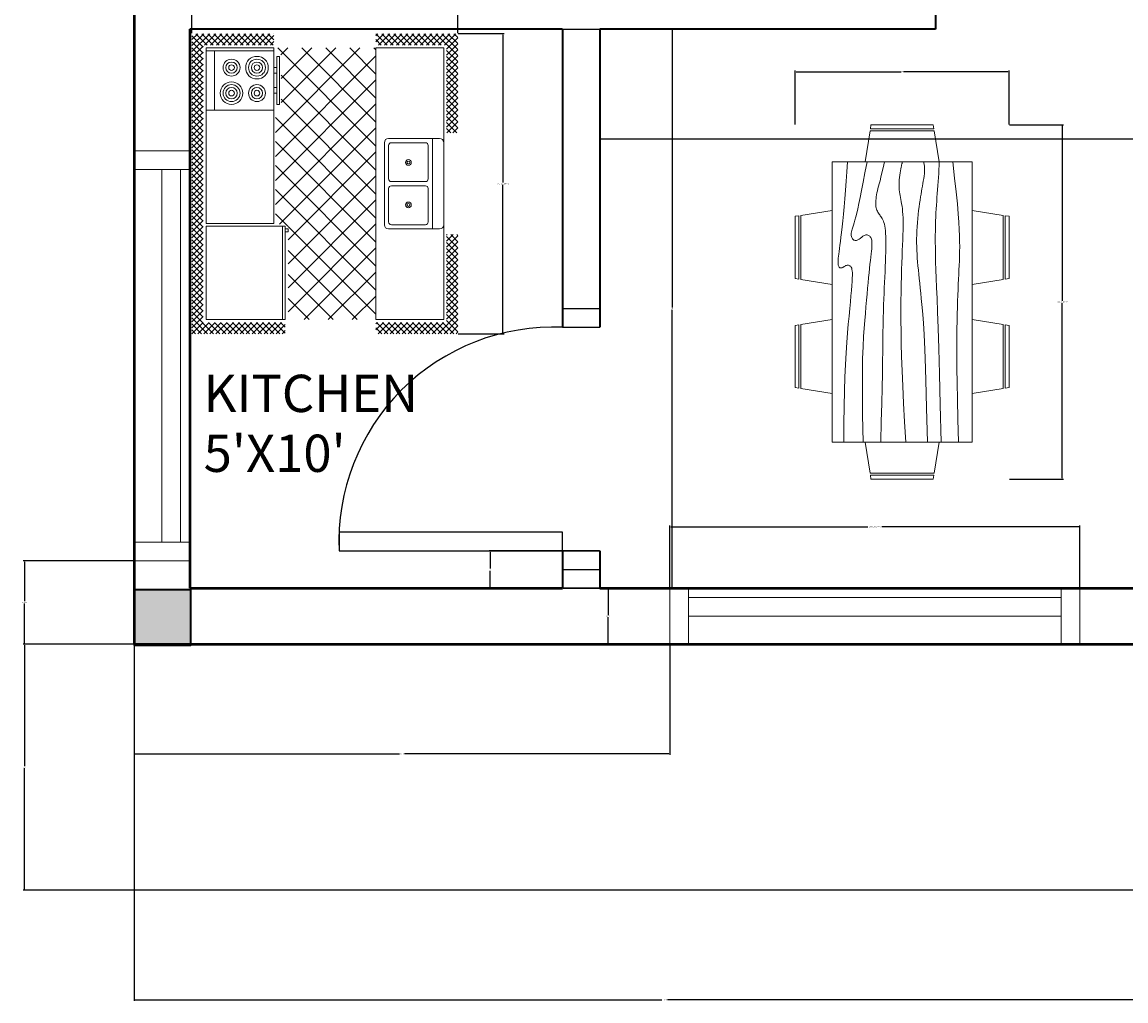
# Model space of a CAD drawing. Units: inches. Extents: x 2421 to 2780, y 382 to 769.
# Tile 1 of 4: x 2421 to 2599, y 382 to 539. Entities that reach past the tile are written whole.
import ezdxf

# ---------------------------------------------------------------- set-up
doc = ezdxf.new("R2010")
doc.units = ezdxf.units.IN
for name, color, linetype, lineweight in [('A-ANNO-DIMS', 2, 'Continuous', 18), ('A-AREA-IDEN', 7, 'Continuous', 25), ('A-COLS', 1, 'Continuous', 35), ('A-FLOR-FIXT', 3, 'Continuous', 18), ('DOOR', 1, 'Continuous', 25), ('FURNITURE', 3, 'Continuous', 18), ('INNER WALL', 2, 'Continuous', 35), ('OUTER WALL', 4, 'Continuous', 50), ('WINDOW', 5, 'Continuous', 18)]:
    doc.layers.add(name, color=color, linetype=linetype, lineweight=lineweight)
doc.styles.get("Standard").update_dxf_attribs({"font": 'arial.ttf'})
doc.dimstyles.get("Standard").update_dxf_attribs({"dimtxt": 0.18, "dimasz": 0.18, "dimexe": 0.18, "dimexo": 0.0625, "dimgap": 0.09, "dimtad": 0, "dimtih": 1, "dimtoh": 1, "dimdec": 4, "dimzin": 0, "dimdsep": 46, "dimtxsty": 'Standard', "dimcen": 0.09, "dimadec": 0, "dimazin": 0, "dimtfac": 1, "dimtdec": 4, "dimtofl": 0, "dimtmove": 0, "dimatfit": 3, "dimfxl": 1, "dimtolj": 1, "dimtzin": 0, "dimarcsym": 0})

# ---------------------------------------------------------------- blocks, each defined once
blk = doc.blocks.new('Dining Set - 36 x 72 in.')
for p, q in [((-22.2343, 26.00059), (-23.4847, 17.99762)), ((-22.2304, 26), (-5.7608, 26)), ((-22, 27.5), (-22.1562, 26.50042)), ((-5.8416, 26.5), (-22.1534, 26.5)), ((-22, 27.5), (-6, 27.5)), ((-5.8437, 26.49966), (-6, 27.5)), ((-4.5152, 17.99762), (-5.7655, 25.99926)), ((5.7657, 26.00059), (4.5153, 17.99762)), ((5.7696, 26), (22.2392, 26)), ((6, 27.5), (5.8438, 26.50042)), ((22.1584, 26.5), (5.8466, 26.5)), ((6, 27.5), (22, 27.5)), ((22.1563, 26.49966), (22, 27.5)), ((23.4848, 17.99762), (22.2345, 25.99926)), ((36, 18), (-36, 18)), ((-36, 18), (-36, -18)), ((36, -18), (36, 18)), ((-44.0006, 8.23428), (-35.9976, 9.48474)), ((44.0006, 8.23428), (35.9976, 9.48474)), ((-45.5, 8), (-44.5004, 8.15617)), ((-45.5, 8), (-45.5, -8)), ((-44.5, -8.15843), (-44.5, 8.15338)), ((-44, 8.23041), (-44, -8.23915)), ((44, 8.23041), (44, -8.23915)), ((44.5, -8.15843), (44.5, 8.15338)), ((45.5, 8), (44.5005, 8.15617)), ((45.5, 8), (45.5, -8)), ((-44.4997, -8.15631), (-45.5, -8)), ((-35.9976, -9.48476), (-43.9993, -8.2345)), ((35.9976, -9.48476), (43.9993, -8.2345)), ((44.4997, -8.15631), (45.5, -8)), ((-36, -18), (36, -18)), ((-22.2343, -26.0006), (-23.4847, -17.99762)), ((-4.5152, -17.99762), (-5.7655, -25.99928)), ((5.7657, -26.0006), (4.5153, -17.99762)), ((23.4848, -17.99762), (22.2345, -25.99928)), ((-22.2304, -26), (-5.7608, -26)), ((-22, -27.5), (-22.1562, -26.50044)), ((-5.8416, -26.5), (-22.1534, -26.5)), ((-22, -27.5), (-6, -27.5)), ((-5.8437, -26.49967), (-6, -27.5)), ((5.7696, -26), (22.2392, -26)), ((6, -27.5), (5.8438, -26.50044)), ((22.1584, -26.5), (5.8466, -26.5)), ((6, -27.5), (22, -27.5)), ((22.1563, -26.49967), (22, -27.5))]:
    blk.add_line(p, q)
for points in [[(-36, 15), (-31.1772, 14.97754), (-26.8079, 14.91406), (-22.8538, 14.81543), (-19.276, 14.6875), (-16.0362, 14.53613), (-13.0957, 14.36718), (-10.4159, 14.18652), (-7.9583, 14), (-5.6904, 13.81315), (-3.6035, 13.63021), (-1.6954, 13.45508), (0.0365, 13.29166), (1.5945, 13.14388), (2.9811, 13.01562), (4.1988, 12.9108), (5.25, 12.83333), (6.1393, 12.78613), (6.8802, 12.76823), (7.4883, 12.77767), (7.9792, 12.8125), (8.3685, 12.87077), (8.6719, 12.95052), (8.9049, 13.0498), (9.0833, 13.16666), (9.2205, 13.29899), (9.3216, 13.44401), (9.3895, 13.59879), (9.4271, 13.76041), (9.4373, 13.92594), (9.4232, 14.09245), (9.3875, 14.257), (9.3333, 14.41666), (9.2638, 14.56917), (9.1836, 14.71484), (9.0975, 14.85465), (9.0104, 14.98958), (8.9272, 15.1206), (8.8529, 15.2487), (8.7922, 15.37483), (8.75, 15.5), (8.7305, 15.62467), (8.7344, 15.74739), (8.7617, 15.86621), (8.8125, 15.97916), (8.8867, 16.08431), (8.9844, 16.17968), (9.1055, 16.26334), (9.25, 16.33333), (9.4189, 16.38802), (9.6172, 16.42708), (9.8506, 16.45052), (10.125, 16.45833), (10.4463, 16.45052), (10.8203, 16.42708), (11.2529, 16.38802), (11.75, 16.33333), (12.3184, 16.26318), (12.9694, 16.17838), (13.7151, 16.07991), (14.5677, 15.96875), (15.5395, 15.84586), (16.6426, 15.71224), (17.8893, 15.56884), (19.2917, 15.41666), (20.859, 15.25667), (22.5879, 15.08984), (24.4721, 14.91715), (26.5052, 14.73958), (28.6809, 14.5581), (30.9929, 14.3737), (33.4347, 14.18733), (36, 14)], [(-36, 10), (-28.9766, 10.14274), (-23.1725, 10.20442), (-18.4241, 10.19775), (-14.5677, 10.13541), (-11.4399, 10.03011), (-8.877, 9.89453), (-6.7154, 9.74137), (-4.7917, 9.58333), (-2.9698, 9.43082), (-1.2246, 9.28515), (0.4415, 9.14534), (2.026, 9.01041), (3.5266, 8.87939), (4.9408, 8.7513), (6.266, 8.62516), (7.5, 8.5), (8.6411, 8.37549), (9.6914, 8.2539), (10.6538, 8.13818), (11.5312, 8.03125), (12.3267, 7.93603), (13.043, 7.85547), (13.6831, 7.79248), (14.25, 7.75), (14.7471, 7.7303), (15.1797, 7.73307), (15.5537, 7.75732), (15.875, 7.80208), (16.1494, 7.86637), (16.3828, 7.94922), (16.5811, 8.04964), (16.75, 8.16666), (16.8944, 8.29915), (17.0143, 8.44531), (17.1089, 8.60319), (17.1771, 8.77083), (17.218, 8.94629), (17.2305, 9.1276), (17.2137, 9.31282), (17.1667, 9.5), (17.0895, 9.6875), (16.987, 9.875), (16.8649, 10.0625), (16.7292, 10.25), (16.5856, 10.4375), (16.4401, 10.625), (16.2985, 10.8125), (16.1667, 11), (16.05, 11.18733), (15.9518, 11.3737), (15.8752, 11.5581), (15.8229, 11.73958), (15.798, 11.91715), (15.8034, 12.08984), (15.842, 12.25667), (15.9167, 12.41666), (16.0295, 12.56836), (16.1784, 12.70833), (16.3605, 12.83268), (16.5729, 12.9375), (16.8127, 13.01888), (17.0768, 13.07291), (17.3625, 13.0957), (17.6667, 13.08333), (17.9894, 13.03312), (18.3418, 12.94726), (18.7382, 12.82918), (19.1927, 12.68229), (19.7195, 12.51001), (20.3327, 12.31575), (21.0465, 12.10294), (21.875, 11.875), (22.8357, 11.63354), (23.959, 11.37304), (25.2786, 11.08618), (26.8282, 10.76562), (28.6414, 10.40405), (30.752, 9.99414), (33.1936, 9.52856), (36, 9)], [(-36, 5.5), (-30.7157, 5.3348), (-26.069, 5.20963), (-21.9946, 5.11767), (-18.4271, 5.05208), (-15.3009, 5.00602), (-12.5508, 4.97265), (-10.1112, 4.94515), (-7.9167, 4.91666), (-5.909, 4.88167), (-4.0586, 4.83984), (-2.3429, 4.79215), (-0.7396, 4.73958), (0.7739, 4.6831), (2.22, 4.6237), (3.6213, 4.56233), (5, 4.5), (6.373, 4.43782), (7.7344, 4.3776), (9.0723, 4.32129), (10.375, 4.27083), (11.6309, 4.22819), (12.8281, 4.19531), (13.9551, 4.17415), (15, 4.16666), (15.954, 4.17448), (16.819, 4.19791), (17.6001, 4.23698), (18.3021, 4.29166), (18.9299, 4.36198), (19.4883, 4.44791), (19.9823, 4.54948), (20.4167, 4.66666), (20.7969, 4.79899), (21.1302, 4.94401), (21.4245, 5.09879), (21.6875, 5.26041), (21.9271, 5.42594), (22.1511, 5.59245), (22.3672, 5.757), (22.5834, 5.91666), (22.8065, 6.06868), (23.0404, 6.21093), (23.2879, 6.34147), (23.5521, 6.45833), (23.8358, 6.55957), (24.142, 6.64323), (24.4735, 6.70735), (24.8334, 6.75), (25.2235, 6.76969), (25.642, 6.76692), (26.0858, 6.74267), (26.5521, 6.69791), (27.0379, 6.63362), (27.5404, 6.55078), (28.0565, 6.45036), (28.5834, 6.33333), (29.1242, 6.19987), (29.7071, 6.04687), (30.3661, 5.87044), (31.1354, 5.66666), (32.0493, 5.43164), (33.142, 5.16146), (34.4475, 4.85221), (36, 4.5)], [(-36, -1), (-30.7915, -0.6591), (-26.0195, -0.38216), (-21.6519, -0.16284), (-17.6563, 0.00521), (-14.0005, 0.12833), (-10.6523, 0.21289), (-7.5796, 0.26522), (-4.75, 0.29166), (-2.134, 0.29793), (0.2878, 0.28711), (2.5317, 0.26163), (4.6146, 0.22396), (6.5529, 0.17651), (8.3633, 0.12174), (10.0623, 0.06209), (11.6667, 0), (13.1899, -0.06201), (14.6341, -0.1211), (15.9982, -0.17432), (17.2813, -0.21875), (18.4823, -0.25147), (19.6003, -0.26953), (20.6343, -0.27002), (21.5834, -0.25), (22.4481, -0.20768), (23.2357, -0.14584), (23.9549, -0.06836), (24.6146, 0.02083), (25.2235, 0.11784), (25.7904, 0.21875), (26.3241, 0.31966), (26.8334, 0.41666), (27.3265, 0.50618), (27.8099, 0.58593), (28.2894, 0.65397), (28.7709, 0.70833), (29.2601, 0.74707), (29.763, 0.76823), (30.2855, 0.76985), (30.8334, 0.75), (31.4088, 0.70784), (31.9994, 0.64713), (32.589, 0.57275), (33.1615, 0.48958), (33.7008, 0.4025), (34.1908, 0.3164), (34.6153, 0.23616), (34.9584, 0.16666), (35.2099, 0.11165), (35.3848, 0.07031), (35.504, 0.04069), (35.5886, 0.02083), (35.6594, 0.00879), (35.7377, 0.0026), (35.8442, 0.00032), (36, 0)], [(-36, -6.5), (-27.1843, -6.31267), (-20.084, -6.1263), (-14.469, -5.9419), (-10.1094, -5.76042), (-6.7752, -5.58285), (-4.2363, -5.41016), (-2.2629, -5.24333), (-0.625, -5.08334), (0.8708, -4.93099), (2.2715, -4.78646), (3.5872, -4.64974), (4.8281, -4.52084), (6.0046, -4.39974), (7.127, -4.28646), (8.2053, -4.18099), (9.25, -4.08334), (10.2705, -3.99382), (11.2734, -3.91407), (12.2647, -3.84603), (13.25, -3.79167), (14.2354, -3.75293), (15.2266, -3.73177), (16.2295, -3.73015), (17.25, -3.75), (18.2912, -3.79248), (19.3451, -3.85547), (20.4009, -3.93604), (21.4479, -4.03125), (22.4754, -4.13819), (23.4727, -4.25391), (24.4289, -4.37549), (25.3334, -4.5), (26.1785, -4.62492), (26.9694, -4.74935), (27.7145, -4.87281), (28.4219, -4.99479), (29.1, -5.11483), (29.7572, -5.23242), (30.4016, -5.34709), (31.0417, -5.45834), (31.6837, -5.56437), (32.3262, -5.65821), (32.9658, -5.73153), (33.599, -5.77604), (34.2224, -5.78345), (34.8327, -5.74545), (35.4264, -5.65373), (36, -5.5)], [(-36, -10), (-26.4022, -9.81299), (-18.4675, -9.62891), (-11.9839, -9.45069), (-6.7396, -9.28125), (-2.5226, -9.12354), (0.8789, -8.98047), (3.6769, -8.85498), (6.0833, -8.75), (8.2767, -8.66765), (10.3021, -8.60677), (12.1712, -8.56543), (13.8958, -8.54167), (15.4876, -8.53353), (16.9583, -8.53907), (18.3197, -8.55632), (19.5834, -8.58334), (20.7616, -8.61841), (21.8685, -8.66081), (22.9188, -8.71004), (23.9271, -8.76563), (24.9081, -8.82707), (25.8763, -8.89388), (26.8465, -8.96558), (27.8334, -9.04167), (28.8474, -9.12118), (29.8828, -9.20117), (30.93, -9.27824), (31.9792, -9.34896), (33.0205, -9.40991), (34.0443, -9.45768), (35.0407, -9.48885), (36, -9.5)], [(-36, -14.5), (-30.0881, -14.33513), (-25.0332, -14.21224), (-20.7312, -14.12647), (-17.0781, -14.07292), (-13.97, -14.04671), (-11.3027, -14.04297), (-8.9724, -14.05681), (-6.875, -14.08334), (-4.9224, -14.11833), (-3.0905, -14.16016), (-1.3709, -14.20785), (0.2448, -14.26042), (1.7647, -14.3169), (3.1973, -14.3763), (4.5507, -14.43767), (5.8333, -14.5), (7.0554, -14.5621), (8.235, -14.62175), (9.3922, -14.67652), (10.5469, -14.72396), (11.7192, -14.76164), (12.929, -14.78711), (14.1965, -14.79794), (15.5417, -14.79167), (16.9933, -14.76424), (18.6152, -14.70508), (20.4804, -14.60197), (22.6615, -14.44271), (25.2312, -14.21509), (28.2624, -13.9069), (31.8277, -13.50594), (36, -13)]]:
    blk.add_lwpolyline(points)
blk = doc.blocks.new('Kitchen Layout - 7 x 8 ft')
for p, q in [((-5, 81.32), (2.68, 89)), ((-5, 83.44), (0.56, 89)), ((-5, 85.56), (-1.56, 89)), ((-5, 87.68), (-3.68, 89)), ((-1, 84.97), (-5, 88.97)), ((-1, 82.85), (-5, 86.85)), ((1.09, 85), (-2.91, 89)), ((3.21, 85), (-0.79, 89)), ((0.81, 85), (4.81, 89)), ((5.34, 85), (1.34, 89)), ((2.93, 85), (6.93, 89)), ((7.46, 85), (3.46, 89)), ((5.05, 85), (9.05, 89)), ((9.58, 85), (5.58, 89)), ((7.17, 85), (11.17, 89)), ((11.7, 85), (7.7, 89)), ((9.29, 85), (13.29, 89)), ((13.82, 85), (9.82, 89)), ((11.41, 85), (15.41, 89)), ((15.94, 85), (11.94, 89)), ((13.53, 85), (17.53, 89)), ((18.06, 85), (14.06, 89)), ((15.65, 85), (19.65, 89)), ((20.18, 85), (16.18, 89)), ((17.78, 85), (21.78, 89)), ((22.31, 85), (18.31, 89)), ((19.9, 85), (23.9, 89)), ((24.43, 85), (20.43, 89)), ((22.02, 85), (26.02, 89)), ((26.55, 85), (22.55, 89)), ((24.14, 85), (28.14, 89)), ((28.67, 85), (24.67, 89)), ((26.26, 85), (30.26, 89)), ((30.79, 85), (26.79, 89)), ((28.38, 85), (32.38, 89)), ((32.91, 85), (28.91, 89)), ((30.5, 85), (34.5, 89)), ((35.03, 85), (31.03, 89)), ((32.63, 85), (36.63, 89)), ((37.16, 85), (33.16, 89)), ((34.75, 85), (38.75, 89)), ((39.28, 85), (35.28, 89)), ((36.87, 85), (40.87, 89)), ((41.4, 85), (37.4, 89)), ((38.99, 85), (42.99, 89)), ((43.52, 85), (39.52, 89)), ((41.11, 85), (45.11, 89)), ((45.64, 85), (41.64, 89)), ((43.23, 85), (47.23, 89)), ((47.76, 85), (43.76, 89)), ((45.35, 85), (49.35, 89)), ((49.88, 85), (45.88, 89)), ((47.47, 85), (51.47, 89)), ((52, 85), (48, 89)), ((49.6, 85), (53.6, 89)), ((54.13, 85), (50.13, 89)), ((51.72, 85), (55.72, 89)), ((56.25, 85), (52.25, 89)), ((53.84, 85), (57.84, 89)), ((58.37, 85), (54.37, 89)), ((55.96, 85), (59.96, 89)), ((60.49, 85), (56.49, 89)), ((58.08, 85), (62.08, 89)), ((62.61, 85), (58.61, 89)), ((60.2, 85), (64.2, 89)), ((64.73, 85), (60.73, 89)), ((62.32, 85), (66.32, 89)), ((66.85, 85), (62.85, 89)), ((64.45, 85), (68.45, 89)), ((68.97, 85), (64.97, 89)), ((66.57, 85), (70.57, 89)), ((71.1, 85), (67.1, 89)), ((68.69, 85), (72.69, 89)), ((73.22, 85), (69.22, 89)), ((70.81, 85), (74.81, 89)), ((75.34, 85), (71.34, 89)), ((72.93, 85), (76.93, 89)), ((77.46, 85), (73.46, 89)), ((75.05, 85), (79.05, 89)), ((79.58, 85), (75.58, 89)), ((77.17, 85), (81.17, 89)), ((81.7, 85), (77.7, 89)), ((79.29, 85), (83.29, 89)), ((83.82, 85), (79.82, 89)), ((81.42, 85), (85.42, 89)), ((85.95, 85), (81.95, 89)), ((83.54, 85), (87.54, 89)), ((88.07, 85), (84.07, 89)), ((85.66, 85), (89.66, 89)), ((90.19, 85), (86.19, 89)), ((87.78, 85), (91.78, 89)), ((92.31, 85), (88.31, 89)), ((89.9, 85), (93.9, 89)), ((94.43, 85), (90.43, 89)), ((92.02, 85), (96.02, 89)), ((96.55, 85), (92.55, 89)), ((94.14, 85), (98.14, 89)), ((101, 82.67), (94.67, 89)), ((96.27, 85), (100.27, 89)), ((101, 84.79), (96.79, 89)), ((97, 83.61), (101, 87.61)), ((101, 86.92), (98.92, 89)), ((-1, 80.73), (-5, 84.73)), ((-5, 79.19), (-1, 83.19)), ((-1, 78.61), (-5, 82.61)), ((34, 84), (96, 84)), ((34, 60), (34, 84)), ((96, 84), (96, 60)), ((97, 81.49), (101, 85.49)), ((101, 80.55), (97, 84.55)), ((97, 79.37), (101, 83.37)), ((101, 78.43), (97, 82.43)), ((-5, 77.07), (-1, 81.07)), ((-1, 76.49), (-5, 80.49)), ((-5, 74.95), (-1, 78.95)), ((-1, 74.36), (-5, 78.36)), ((74, 81), (95, 81)), ((97, 77.25), (101, 81.25)), ((101, 76.31), (97, 80.31)), ((97, 75.13), (101, 79.13)), ((101, 74.19), (97, 78.19)), ((-5, 72.83), (-1, 76.83)), ((-1, 72.24), (-5, 76.24)), ((-5, 70.71), (-1, 74.71)), ((-1, 70.12), (-5, 74.12)), ((97, 73.01), (101, 77.01)), ((101, 72.07), (97, 76.07)), ((97, 70.89), (101, 74.89)), ((-5, 68.59), (-1, 72.59)), ((-1, 68), (-5, 72)), ((-5, 66.47), (-1, 70.47)), ((101, 69.95), (97, 73.95)), ((97, 68.76), (101, 72.76)), ((101, 67.82), (97, 71.82)), ((97, 66.64), (101, 70.64)), ((-1, 65.88), (-5, 69.88)), ((-5, 64.35), (-1, 68.35)), ((-1, 63.76), (-5, 67.76)), ((101, 65.7), (97, 69.7)), ((97, 64.52), (101, 68.52)), ((101, 63.58), (97, 67.58)), ((97, 62.4), (101, 66.4)), ((-5, 62.22), (-1, 66.22)), ((-1, 61.64), (-5, 65.64)), ((-5, 60.1), (-1, 64.1)), ((-1, 59.52), (-5, 63.52)), ((101, 61.46), (97, 65.46)), ((97, 60.28), (101, 64.28)), ((100.34, 60), (97, 63.34)), ((-5, 57.98), (-1, 61.98)), ((-1, 57.39), (-5, 61.39)), ((-1.73, 56), (-5, 59.27)), ((-4.86, 56), (-1, 59.86)), ((10.4, 24), (45.9, 59.5)), ((18.88, 24), (54.38, 59.5)), ((27.37, 24), (62.87, 59.5)), ((33.03, 55.11), (37.41, 59.5)), ((96, 60), (34, 60)), ((35.85, 24), (71.35, 59.5)), ((76.2, 24), (40.7, 59.5)), ((84.68, 24), (49.18, 59.5)), ((93.17, 24), (57.67, 59.5)), ((61.31, 24), (96, 58.69)), ((96, 29.65), (66.15, 59.5)), ((80, 60), (80, 59)), ((82, 59), (82, 60)), ((87, 59), (87, 60)), ((89, 60), (89, 59)), ((98.22, 60), (97, 61.22)), ((98.84, 60), (101, 62.16)), ((100.96, 60), (101, 60.04)), ((-3.85, 56), (-5, 57.15)), ((-2.74, 56), (-1, 57.74)), ((0, 57), (33, 57)), ((0, 30.57), (24.43, 55)), ((0, 39.06), (15.94, 55)), ((0, 47.54), (7.46, 55)), ((1.91, 24), (32.91, 55)), ((33.77, 24), (2.77, 55)), ((42.26, 24), (11.26, 55)), ((50.74, 24), (19.74, 55)), ((59.23, 24), (28.23, 55)), ((31, 55), (31, 56)), ((32, 55), (31, 55)), ((32, 56), (32, 55)), ((67.71, 24), (33.68, 58.04)), ((44.34, 24), (77.84, 57.5)), ((52.82, 24), (86.32, 57.5)), ((96, 38.14), (76.64, 57.5)), ((96, 46.63), (85.13, 57.5)), ((96, 55.11), (93.57, 57.54)), ((25.29, 24), (0, 49.29)), ((69.79, 24), (96, 50.21)), ((16.8, 24), (0, 40.8)), ((78.28, 24), (96, 41.72)), ((8.32, 24), (0, 32.32)), ((86.76, 24), (96, 33.24)), ((-5, 21.92), (-2.92, 24)), ((-5, 19.8), (-1, 23.8)), ((-1, 21.33), (-3.67, 24)), ((-1, 23.45), (-1.55, 24)), ((0, 24), (96, 24)), ((0, 0), (0, 24)), ((95.25, 24), (96, 24.75)), ((96, 24), (96, 0)), ((97, 22.1), (98.9, 24)), ((97, 19.97), (101, 23.97)), ((101, 21.16), (98.16, 24)), ((101, 23.28), (100.28, 24)), ((-1, 19.21), (-5, 23.21)), ((-5, 17.68), (-1, 21.68)), ((-1, 17.09), (-5, 21.09)), ((-5, 15.55), (-1, 19.55)), ((101, 19.03), (97, 23.03)), ((97, 17.85), (101, 21.85)), ((101, 16.91), (97, 20.91)), ((97, 15.73), (101, 19.73)), ((-1, 14.97), (-5, 18.97)), ((-5, 13.43), (-1, 17.43)), ((-1, 12.85), (-5, 16.85)), ((47.25, 6.5), (47.25, 18.5)), ((48.75, 18.5), (48.75, 6.5)), ((101, 14.79), (97, 18.79)), ((97, 13.61), (101, 17.61)), ((101, 12.67), (97, 16.67)), ((-5, 11.31), (-1, 15.31)), ((-1, 10.73), (-5, 14.73)), ((-5, 9.19), (-1, 13.19)), ((-1, 8.6), (-5, 12.6)), ((97, 11.49), (101, 15.49)), ((101, 10.55), (97, 14.55)), ((97, 9.37), (101, 13.37)), ((101, 8.43), (97, 12.43)), ((-5, 7.07), (-1, 11.07)), ((-1, 6.48), (-5, 10.48)), ((-5, 4.95), (-1, 8.95)), ((-1, 4.36), (-5, 8.36)), ((97, 7.25), (101, 11.25)), ((101, 6.31), (97, 10.31)), ((97, 5.12), (101, 9.12)), ((101, 4.18), (97, 8.18)), ((-5, 2.83), (-1, 6.83)), ((-1, 2.24), (-5, 6.24)), ((-5, 0.71), (-1, 4.71)), ((-1, 0.12), (-5, 4.12)), ((64, 4), (32, 4)), ((97, 3), (101, 7)), ((101, 2.06), (97, 6.06)), ((97, 0.88), (101, 4.88)), ((101, -0.06), (97, 3.94)), ((-5, -1.42), (-1, 2.58)), ((2, -5), (-5, 2)), ((-5, -3.54), (-1, 0.46)), ((96, 0), (0, 0)), ((93.24, -5), (101, 2.76)), ((95.36, -5), (101, 0.64)), ((101, -2.18), (97, 1.82)), ((-0.12, -5), (-5, -0.12)), ((-2.25, -5), (-5, -2.25)), ((-4.34, -5), (-0.34, -1)), ((-2.22, -5), (1.78, -1)), ((-0.1, -5), (3.9, -1)), ((4.12, -5), (0.12, -1)), ((2.02, -5), (6.02, -1)), ((6.24, -5), (2.24, -1)), ((4.14, -5), (8.14, -1)), ((8.36, -5), (4.36, -1)), ((6.27, -5), (10.27, -1)), ((10.48, -5), (6.48, -1)), ((8.39, -5), (12.39, -1)), ((12.6, -5), (8.6, -1)), ((10.51, -5), (14.51, -1)), ((14.73, -5), (10.73, -1)), ((12.63, -5), (16.63, -1)), ((16.85, -5), (12.85, -1)), ((14.75, -5), (18.75, -1)), ((18.97, -5), (14.97, -1)), ((16.87, -5), (20.87, -1)), ((21.09, -5), (17.09, -1)), ((18.99, -5), (22.99, -1)), ((23.21, -5), (19.21, -1)), ((21.11, -5), (25.11, -1)), ((25.33, -5), (21.33, -1)), ((23.24, -5), (27.24, -1)), ((27.45, -5), (23.45, -1)), ((25.36, -5), (29.36, -1)), ((29.57, -5), (25.57, -1)), ((27.48, -5), (30, -2.48)), ((30, -3.3), (27.7, -1)), ((30, -1.18), (29.82, -1)), ((66, -2.54), (67.54, -1)), ((66, -4.66), (69.66, -1)), ((69.88, -5), (66, -1.12)), ((67.76, -5), (66, -3.24)), ((67.78, -5), (71.78, -1)), ((72, -5), (68, -1)), ((69.9, -5), (73.9, -1)), ((74.12, -5), (70.12, -1)), ((72.03, -5), (76.03, -1)), ((76.24, -5), (72.24, -1)), ((74.15, -5), (78.15, -1)), ((78.36, -5), (74.36, -1)), ((76.27, -5), (80.27, -1)), ((80.49, -5), (76.49, -1)), ((78.39, -5), (82.39, -1)), ((82.61, -5), (78.61, -1)), ((80.51, -5), (84.51, -1)), ((84.73, -5), (80.73, -1)), ((82.63, -5), (86.63, -1)), ((86.85, -5), (82.85, -1)), ((84.75, -5), (88.75, -1)), ((88.97, -5), (84.97, -1)), ((86.88, -5), (90.88, -1)), ((91.09, -5), (87.09, -1)), ((89, -5), (93, -1)), ((93.21, -5), (89.21, -1)), ((91.12, -5), (95.12, -1)), ((95.34, -5), (91.34, -1)), ((97.46, -5), (93.46, -1)), ((99.58, -5), (95.58, -1)), ((101, -4.3), (97, -0.3)), ((97.48, -5), (101, -1.48)), ((99.6, -5), (101, -3.6)), ((-4.37, -5), (-5, -4.37)), ((29.6, -5), (30, -4.6))]:
    blk.add_line(p, q)
for points in [[(0, 56), (0, 84), (33, 84), (33, 56)], [(74, 60), (74, 84), (95, 84), (95, 60)], [(76, 58), (76, 59), (93, 59), (93, 58)]]:
    blk.add_lwpolyline(points, close=True)
for points in [[(33.5, 21), (62.5, 21)], [(32, 1.5), (32, 19.5)], [(33.5, 6.5), (33.5, 18.5)], [(34.5, 19.5), (46.25, 19.5)], [(49.75, 19.5), (61.5, 19.5)], [(62.5, 18.5), (62.5, 6.5)], [(64, 19.5), (64, 1.5)], [(46.25, 5.5), (34.5, 5.5)], [(61.5, 5.5), (49.75, 5.5)], [(62.5, 0), (33.5, 0)]]:
    blk.add_lwpolyline(points)
for centre, radius in [((80, 75), 4), ((80, 75), 3), ((80, 75), 2), ((80, 75), 1), ((89, 75), 3), ((89, 75), 2), ((89, 75), 1), ((80, 66), 3), ((80, 66), 2), ((80, 66), 1), ((89, 66), 4), ((89, 66), 3), ((89, 66), 2), ((89, 66), 1), ((40.5, 12.5), 1), ((40.5, 12.5), 0.5), ((55.5, 12.5), 1), ((55.5, 12.5), 0.5)]:
    blk.add_circle(centre, radius)
for centre, radius, start, end in [((33.5, 19.5), 1.5, 90, 180), ((62.5, 19.5), 1.5, 0, 90), ((34.5, 18.5), 1, 90, 180), ((46.25, 18.5), 1, 0, 90), ((49.75, 18.5), 1, 90, 180), ((61.5, 18.5), 1, 0, 90), ((34.5, 6.5), 1, 180, 270), ((46.25, 6.5), 1, 270, 0), ((49.75, 6.5), 1, 180, 270), ((61.5, 6.5), 1, 270, 0), ((33.5, 1.5), 1.5, 180, 270), ((62.5, 1.5), 1.5, 270, 0)]:
    blk.add_arc(centre, radius, start, end)
blk = doc.blocks.new('DOOR-36IN-INT')
for p, q in [((0, 6), (0, 0)), ((3, 6), (3, 0)), ((39, 6), (39, 0)), ((42, 6), (42, 0))]:
    blk.add_line(p, q)
blk.add_lwpolyline([(3, 6), (6, 6), (6, 42), (3, 42)], close=True)
blk.add_arc((4.5, 7.5), 34.53, 357.5104, 92.4896)
blk = doc.blocks.new('WIN-60IN')
for p, q in [((0, 0), (0, 9)), ((3, 0), (3, 9)), ((63, 9), (63, 0)), ((66, 9), (66, 0)), ((63, 4.5), (3, 4.5)), ((63, 1.5), (3, 1.5))]:
    blk.add_line(p, q)
blk = doc.blocks.new('COL-9X9IN')
h = blk.add_hatch(color=256)
h.dxf.hatch_style = 1
h.paths.add_polyline_path([(9, 9), (0, 9), (0, 0), (9, 0)])
blk.add_lwpolyline([(0, 9), (9, 9), (9, 0), (0, 0)], close=True)
blk = doc.blocks.new('*D20')
at = {"layer": 'A-ANNO-DIMS', "color": 0, "lineweight": -2, "transparency": 16777216}
for p, q in [((2525.72, 448.24), (2525.72, 458.26)), ((2525.9, 458.08), (2557.6, 458.08)), ((2591.54, 458.08), (2559.84, 458.08)), ((2591.72, 448.24), (2591.72, 458.26))]:
    blk.add_line(p, q, dxfattribs=at)
at = {"layer": 'A-ANNO-DIMS', "color": 0, "transparency": 16777216}
for points in [[(2525.9, 458.11), (2525.9, 458.05), (2525.72, 458.08)], [(2591.54, 458.11), (2591.54, 458.05), (2591.72, 458.08)]]:
    blk.add_solid(points, dxfattribs=at)
at = {"layer": 'Defpoints', "color": 0, "transparency": 16777216}
for p in [(2525.72, 458.08), (2525.72, 448.18), (2591.72, 448.18)]:
    blk.add_point(p, dxfattribs=at)
at = {"layer": 'A-ANNO-DIMS', "color": 0, "transparency": 16777216, "insert": (2558.72, 458.08), "char_height": 0.18, "attachment_point": 5}
blk.add_mtext('\\A1;WINDOW 66 TYP.', dxfattribs=at)
blk = doc.blocks.new('*D21')
at = {"layer": 'A-ANNO-DIMS', "color": 0, "lineweight": -2, "transparency": 16777216}
for p, q in [((2525.66, 448.18), (2515.64, 448.18)), ((2515.82, 448), (2515.82, 443.86)), ((2515.82, 439.36), (2515.82, 443.5)), ((2525.66, 439.18), (2515.64, 439.18))]:
    blk.add_line(p, q, dxfattribs=at)
at = {"layer": 'A-ANNO-DIMS', "color": 0, "transparency": 16777216}
for points in [[(2515.79, 448), (2515.85, 448), (2515.82, 448.18)], [(2515.79, 439.36), (2515.85, 439.36), (2515.82, 439.18)]]:
    blk.add_solid(points, dxfattribs=at)
at = {"layer": 'Defpoints', "color": 0, "transparency": 16777216}
for p in [(2525.72, 448.18), (2515.82, 439.18), (2525.72, 439.18)]:
    blk.add_point(p, dxfattribs=at)
at = {"layer": 'A-ANNO-DIMS', "color": 0, "transparency": 16777216, "insert": (2515.82, 443.68), "char_height": 0.18, "attachment_point": 5}
blk.add_mtext('\\A1;9 TYP.', dxfattribs=at)
blk = doc.blocks.new('*D42')
at = {"layer": 'A-ANNO-DIMS', "color": 0, "lineweight": -2, "transparency": 16777216}
for p, q in [((2580.41, 522.76), (2589.08, 522.76)), ((2588.9, 522.58), (2588.9, 494.44)), ((2588.9, 465.92), (2588.9, 494.07)), ((2580.41, 465.74), (2589.08, 465.74))]:
    blk.add_line(p, q, dxfattribs=at)
at = {"layer": 'A-ANNO-DIMS', "color": 0, "transparency": 16777216}
for points in [[(2588.87, 522.58), (2588.93, 522.58), (2588.9, 522.76)], [(2588.87, 465.92), (2588.93, 465.92), (2588.9, 465.74)]]:
    blk.add_solid(points, dxfattribs=at)
at = {"layer": 'Defpoints', "color": 0, "transparency": 16777216}
for p in [(2580.34, 522.76), (2588.9, 522.76), (2580.34, 465.74)]:
    blk.add_point(p, dxfattribs=at)
at = {"layer": 'A-ANNO-DIMS', "color": 0, "transparency": 16777216, "insert": (2588.9, 494.25), "char_height": 0.18, "attachment_point": 5}
blk.add_mtext('\\A1;DINING SET 57', dxfattribs=at)
blk = doc.blocks.new('*D43')
at = {"layer": 'A-ANNO-DIMS', "color": 0, "lineweight": -2, "transparency": 16777216}
for p, q in [((2545.88, 522.83), (2545.88, 531.5)), ((2580.34, 522.83), (2580.34, 531.5)), ((2546.06, 531.32), (2562.89, 531.32)), ((2580.16, 531.32), (2563.33, 531.32))]:
    blk.add_line(p, q, dxfattribs=at)
at = {"layer": 'A-ANNO-DIMS', "color": 0, "transparency": 16777216}
for points in [[(2546.06, 531.35), (2546.06, 531.29), (2545.88, 531.32)], [(2580.16, 531.35), (2580.16, 531.29), (2580.34, 531.32)]]:
    blk.add_solid(points, dxfattribs=at)
at = {"layer": 'Defpoints', "color": 0, "transparency": 16777216}
for p in [(2545.88, 531.32), (2545.88, 522.76), (2580.34, 522.76)]:
    blk.add_point(p, dxfattribs=at)
at = {"layer": 'A-ANNO-DIMS', "color": 0, "transparency": 16777216, "insert": (2563.11, 531.32), "char_height": 0.18, "attachment_point": 5}
blk.add_mtext('\\A1;34', dxfattribs=at)
blk = doc.blocks.new('*D44')
at = {"layer": 'A-ANNO-DIMS', "color": 0, "lineweight": -2, "transparency": 16777216}
for p, q in [((2491.67, 537.44), (2499.03, 537.44)), ((2498.85, 537.26), (2498.85, 513.47)), ((2498.85, 489.32), (2498.85, 513.11)), ((2491.67, 489.14), (2499.03, 489.14))]:
    blk.add_line(p, q, dxfattribs=at)
at = {"layer": 'A-ANNO-DIMS', "color": 0, "transparency": 16777216}
for points in [[(2498.82, 537.26), (2498.88, 537.26), (2498.85, 537.44)], [(2498.82, 489.32), (2498.88, 489.32), (2498.85, 489.14)]]:
    blk.add_solid(points, dxfattribs=at)
at = {"layer": 'Defpoints', "color": 0, "transparency": 16777216}
for p in [(2491.61, 537.44), (2498.85, 537.44), (2491.61, 489.14)]:
    blk.add_point(p, dxfattribs=at)
at = {"layer": 'A-ANNO-DIMS', "color": 0, "transparency": 16777216, "insert": (2498.85, 513.29), "char_height": 0.18, "attachment_point": 5}
blk.add_mtext('\\A1;KITCHEN UNIT 48', dxfattribs=at)
blk = doc.blocks.new('*D45')
at = {"layer": 'A-ANNO-DIMS', "color": 0, "lineweight": -2, "transparency": 16777216}
for p, q in [((2448.78, 537.5), (2448.78, 544.86)), ((2448.96, 544.68), (2469.97, 544.68)), ((2491.43, 544.68), (2470.42, 544.68)), ((2491.61, 537.5), (2491.61, 544.86))]:
    blk.add_line(p, q, dxfattribs=at)
at = {"layer": 'A-ANNO-DIMS', "color": 0, "transparency": 16777216}
for points in [[(2448.96, 544.71), (2448.96, 544.65), (2448.78, 544.68)], [(2491.43, 544.71), (2491.43, 544.65), (2491.61, 544.68)]]:
    blk.add_solid(points, dxfattribs=at)
at = {"layer": 'Defpoints', "color": 0, "transparency": 16777216}
for p in [(2448.78, 544.68), (2448.78, 537.44), (2491.61, 537.44)]:
    blk.add_point(p, dxfattribs=at)
at = {"layer": 'A-ANNO-DIMS', "color": 0, "transparency": 16777216, "insert": (2470.19, 544.68), "char_height": 0.18, "attachment_point": 5}
blk.add_mtext('\\A1;43', dxfattribs=at)
blk = doc.blocks.new('*D49')
at = {"layer": 'A-ANNO-DIMS', "color": 0, "lineweight": -2, "transparency": 16777216}
for p, q in [((2439.47, 439.12), (2439.47, 381.75)), ((2610.35, 439.12), (2610.35, 381.75)), ((2439.65, 381.93), (2524.45, 381.93)), ((2610.17, 381.93), (2525.36, 381.93))]:
    blk.add_line(p, q, dxfattribs=at)
at = {"layer": 'A-ANNO-DIMS', "color": 0, "transparency": 16777216}
for points in [[(2439.65, 381.96), (2439.65, 381.9), (2439.47, 381.93)], [(2610.17, 381.96), (2610.17, 381.9), (2610.35, 381.93)]]:
    blk.add_solid(points, dxfattribs=at)
at = {"layer": 'Defpoints', "color": 0, "transparency": 16777216}
for p in [(2439.47, 439.18), (2610.35, 439.18), (2610.35, 381.93)]:
    blk.add_point(p, dxfattribs=at)
at = {"layer": 'A-ANNO-DIMS', "color": 0, "transparency": 16777216, "insert": (2524.91, 381.93), "char_height": 0.18, "attachment_point": 5}
blk.add_mtext('\\A1;170.88', dxfattribs=at)
blk = doc.blocks.new('*D50')
at = {"layer": 'A-ANNO-DIMS', "color": 0, "lineweight": -2, "transparency": 16777216}
for p, q in [((2439.4, 439.18), (2421.64, 439.18)), ((2421.82, 439), (2421.82, 419.56)), ((2421.82, 399.76), (2421.82, 419.2)), ((2610.28, 399.58), (2421.64, 399.58))]:
    blk.add_line(p, q, dxfattribs=at)
at = {"layer": 'A-ANNO-DIMS', "color": 0, "transparency": 16777216}
for points in [[(2421.79, 439), (2421.85, 439), (2421.82, 439.18)], [(2421.79, 399.76), (2421.85, 399.76), (2421.82, 399.58)]]:
    blk.add_solid(points, dxfattribs=at)
at = {"layer": 'Defpoints', "color": 0, "transparency": 16777216}
for p in [(2421.82, 439.18), (2439.47, 439.18), (2610.35, 399.58)]:
    blk.add_point(p, dxfattribs=at)
at = {"layer": 'A-ANNO-DIMS', "color": 0, "transparency": 16777216, "insert": (2421.82, 419.38), "char_height": 0.18, "attachment_point": 5}
blk.add_mtext('\\A1;39.6', dxfattribs=at)
blk = doc.blocks.new('*D51')
at = {"layer": 'A-ANNO-DIMS', "color": 0, "lineweight": -2, "transparency": 16777216}
for p, q in [((2508.53, 538.18), (2526.3, 538.18)), ((2526.12, 538), (2526.12, 493.36)), ((2526.12, 448.36), (2526.12, 493)), ((2508.53, 448.18), (2526.3, 448.18))]:
    blk.add_line(p, q, dxfattribs=at)
at = {"layer": 'A-ANNO-DIMS', "color": 0, "transparency": 16777216}
for points in [[(2526.09, 538), (2526.15, 538), (2526.12, 538.18)], [(2526.09, 448.36), (2526.15, 448.36), (2526.12, 448.18)]]:
    blk.add_solid(points, dxfattribs=at)
at = {"layer": 'Defpoints', "color": 0, "transparency": 16777216}
for p in [(2508.47, 538.18), (2508.47, 448.18), (2526.12, 448.18)]:
    blk.add_point(p, dxfattribs=at)
at = {"layer": 'A-ANNO-DIMS', "color": 0, "transparency": 16777216, "insert": (2526.12, 493.18), "char_height": 0.18, "attachment_point": 5}
blk.add_mtext('\\A1;90', dxfattribs=at)
blk = doc.blocks.new('*D54')
at = {"layer": 'A-ANNO-DIMS', "color": 0, "lineweight": -2, "transparency": 16777216}
for p, q in [((2514.47, 538.12), (2514.47, 520.35)), ((2742.47, 538.12), (2742.47, 520.35)), ((2514.65, 520.53), (2628.18, 520.53)), ((2742.29, 520.53), (2628.76, 520.53))]:
    blk.add_line(p, q, dxfattribs=at)
at = {"layer": 'A-ANNO-DIMS', "color": 0, "transparency": 16777216}
for points in [[(2514.65, 520.56), (2514.65, 520.5), (2514.47, 520.53)], [(2742.29, 520.56), (2742.29, 520.5), (2742.47, 520.53)]]:
    blk.add_solid(points, dxfattribs=at)
at = {"layer": 'Defpoints', "color": 0, "transparency": 16777216}
for p in [(2514.47, 538.18), (2742.47, 538.18), (2514.47, 520.53)]:
    blk.add_point(p, dxfattribs=at)
at = {"layer": 'A-ANNO-DIMS', "color": 0, "transparency": 16777216, "insert": (2628.47, 520.53), "char_height": 0.18, "attachment_point": 5}
blk.add_mtext('\\A1;228', dxfattribs=at)
blk = doc.blocks.new('*D61')
at = {"layer": 'A-ANNO-DIMS', "color": 0, "lineweight": -2, "transparency": 16777216}
for p, q in [((2439.4, 452.6), (2421.64, 452.6)), ((2421.82, 452.42), (2421.82, 446.07)), ((2421.82, 439.36), (2421.82, 445.71)), ((2439.4, 439.18), (2421.64, 439.18))]:
    blk.add_line(p, q, dxfattribs=at)
at = {"layer": 'A-ANNO-DIMS', "color": 0, "transparency": 16777216}
for points in [[(2421.79, 452.42), (2421.85, 452.42), (2421.82, 452.6)], [(2421.79, 439.36), (2421.85, 439.36), (2421.82, 439.18)]]:
    blk.add_solid(points, dxfattribs=at)
at = {"layer": 'Defpoints', "color": 0, "transparency": 16777216}
for p in [(2421.82, 452.6), (2439.47, 452.6), (2439.47, 439.18)]:
    blk.add_point(p, dxfattribs=at)
at = {"layer": 'A-ANNO-DIMS', "color": 0, "transparency": 16777216, "insert": (2421.82, 445.89), "char_height": 0.18, "attachment_point": 5}
blk.add_mtext('\\A1;13.418', dxfattribs=at)
blk = doc.blocks.new('*D64')
at = {"layer": 'A-ANNO-DIMS', "color": 0, "lineweight": -2, "transparency": 16777216}
for p, q in [((2439.47, 439.12), (2439.47, 421.35)), ((2525.72, 439.12), (2525.72, 421.35)), ((2439.65, 421.53), (2482.2, 421.53)), ((2525.54, 421.53), (2482.99, 421.53))]:
    blk.add_line(p, q, dxfattribs=at)
at = {"layer": 'A-ANNO-DIMS', "color": 0, "transparency": 16777216}
for points in [[(2439.65, 421.56), (2439.65, 421.5), (2439.47, 421.53)], [(2525.54, 421.56), (2525.54, 421.5), (2525.72, 421.53)]]:
    blk.add_solid(points, dxfattribs=at)
at = {"layer": 'Defpoints', "color": 0, "transparency": 16777216}
for p in [(2439.47, 439.18), (2525.72, 439.18), (2439.47, 421.53)]:
    blk.add_point(p, dxfattribs=at)
at = {"layer": 'A-ANNO-DIMS', "color": 0, "transparency": 16777216, "insert": (2482.59, 421.53), "char_height": 0.18, "attachment_point": 5}
blk.add_mtext('\\A1;86.26', dxfattribs=at)
blk = doc.blocks.new('*D69')
at = {"layer": 'A-ANNO-DIMS', "color": 0, "lineweight": -2, "transparency": 16777216}
for p, q in [((2514.4, 454.18), (2496.64, 454.18)), ((2496.82, 454), (2496.82, 451.36)), ((2496.82, 448.36), (2496.82, 451)), ((2514.4, 448.18), (2496.64, 448.18))]:
    blk.add_line(p, q, dxfattribs=at)
at = {"layer": 'A-ANNO-DIMS', "color": 0, "transparency": 16777216}
for points in [[(2496.79, 454), (2496.85, 454), (2496.82, 454.18)], [(2496.79, 448.36), (2496.85, 448.36), (2496.82, 448.18)]]:
    blk.add_solid(points, dxfattribs=at)
at = {"layer": 'Defpoints', "color": 0, "transparency": 16777216}
for p in [(2496.82, 454.18), (2514.47, 454.18), (2514.47, 448.18)]:
    blk.add_point(p, dxfattribs=at)
at = {"layer": 'A-ANNO-DIMS', "color": 0, "transparency": 16777216, "insert": (2496.82, 451.18), "char_height": 0.18, "attachment_point": 5}
blk.add_mtext('\\A1;6', dxfattribs=at)

msp = doc.modelspace()

# ---------------------------------------------------------------- linework, layer by layer
at = {"layer": 'INNER WALL'}
for p, q in [((2568.466, 592.1806), (2568.466, 538.1806)), ((2508.466, 538.1806), (2448.466, 538.1806)), ((2508.466, 538.1806), (2508.466, 490.1806)), ((2568.466, 538.1806), (2514.466, 538.1806)), ((2514.466, 538.1806), (2514.466, 490.1806)), ((2508.466, 454.1806), (2508.466, 448.1806)), ((2514.466, 454.1806), (2514.466, 448.1806))]:
    msp.add_line(p, q, dxfattribs=at)
at = {"layer": 'OUTER WALL'}
for p, q in [((2448.466, 538.1806), (2448.466, 448.1806)), ((2448.466, 448.1806), (2508.466, 448.1806)), ((2514.466, 448.1806), (2620.7381, 448.1806))]:
    msp.add_line(p, q, dxfattribs=at)
msp.add_lwpolyline([(2656.7381, 439.1806), (2751.466, 439.1806), (2751.466, 751.1806), (2439.466, 751.1806), (2439.466, 439.1806), (2620.7381, 439.1806)], dxfattribs=at)
at = {"layer": 'WINDOW'}
for p, q in [((2528.723, 448.1806), (2588.723, 448.1806)), ((2588.723, 439.1806), (2528.723, 439.1806))]:
    msp.add_line(p, q, dxfattribs=at)

# ---------------------------------------------------------------- block references
at = {"layer": 'A-COLS'}
msp.add_blockref('COL-9X9IN', (2439.5377, 438.9565), dxfattribs=at)
at = {"layer": 'A-FLOR-FIXT', "xscale": 0.4555841685436928, "yscale": 0.4555841685436928, "zscale": 0.4555841685436928, "rotation": 90}
msp.add_blockref('Kitchen Layout - 7 x 8 ft', (2489.3289, 491.4212), dxfattribs=at)
at = {"layer": 'DOOR', "rotation": 89.99999999999812}
msp.add_blockref('DOOR-36IN-INT', (2514.466, 451.1806), dxfattribs=at)
at = {"layer": 'FURNITURE', "xscale": 0.6266177380720624, "yscale": 0.6266177380720624, "zscale": 0.6266177380720624, "rotation": 90}
msp.add_blockref('Dining Set - 36 x 72 in.', (2563.1126, 494.2529), dxfattribs=at)
at = {"layer": 'WINDOW'}
for p, rotation in [((2448.466, 452.5986), 89.99999999999989), ((2591.723, 448.1806), 180)]:
    msp.add_blockref('WIN-60IN', p, dxfattribs=dict(at, rotation=rotation))

# ---------------------------------------------------------------- texts
at = {"layer": 'A-AREA-IDEN'}
for s, p in [('KITCHEN', (2450.6706, 476.5394)), ("5'X10'", (2450.6706, 466.9009))]:
    msp.add_text(s, height=6, dxfattribs=at).set_placement(p)

# ---------------------------------------------------------------- dimensions: what is measured, and where the dimension line sits
at = {"layer": 'A-ANNO-DIMS'}
for base, p1, p2, angle, override, picture, middle in [((2448.7819, 544.679), (2491.6068, 537.4352), (2448.7819, 537.4352), 180, {"dimdec": 0, "dimlfac": 1, "dimrnd": 0, "dimzin": 0, "dimdsep": 46, "dimlunit": 2}, '*D45', (2470.1943, 544.679)), ((2526.116, 448.1806), (2508.466, 538.1806), (2508.466, 448.1806), 270, {"dimdec": 0, "dimlfac": 1, "dimrnd": 0, "dimzin": 0, "dimdsep": 46, "dimlunit": 2}, '*D51', (2526.116, 493.1806)), ((2514.466, 520.5306), (2742.466, 538.1806), (2514.466, 538.1806), 180, {"dimdec": 0, "dimlfac": 1, "dimrnd": 0, "dimzin": 0, "dimdsep": 46, "dimlunit": 2}, '*D54', (2628.466, 520.5306)), ((2545.8806, 531.3173), (2580.3445, 522.764), (2545.8806, 522.764), 180, {"dimdec": 0, "dimlfac": 1, "dimrnd": 0, "dimzin": 0, "dimdsep": 46, "dimlunit": 2}, '*D43', (2563.1126, 531.3173)), ((2496.816, 454.1806), (2514.466, 448.1806), (2514.466, 454.1806), 90, {"dimdec": 0, "dimlfac": 1, "dimrnd": 0, "dimzin": 0, "dimdsep": 46, "dimlunit": 2}, '*D69', (2496.816, 451.1806)), ((2421.816, 452.5986), (2439.466, 439.1806), (2439.466, 452.5986), 90, {"dimdec": 3, "dimlfac": 1, "dimrnd": 0, "dimzin": 0, "dimdsep": 46, "dimlunit": 2}, '*D61', (2421.816, 445.8896)), ((2421.816, 439.1806), (2610.347, 399.5831), (2439.466, 439.1806), 90, {"dimdec": 1, "dimlfac": 1, "dimrnd": 0, "dimzin": 0, "dimdsep": 46, "dimlunit": 2}, '*D50', (2421.816, 419.3818)), ((2439.466, 421.5306), (2525.723, 439.1806), (2439.466, 439.1806), 180, {"dimdec": 2, "dimlfac": 1, "dimrnd": 0, "dimzin": 0, "dimdsep": 46, "dimlunit": 2}, '*D64', (2482.5945, 421.5306))]:
    dim = msp.add_linear_dim(base=base, p1=p1, p2=p2, angle=angle, dimstyle='Standard', override=override, dxfattribs=at)
    dim.commit()
    dim.dimension.update_dxf_attribs({"geometry": picture, "text_midpoint": middle})
for base, p1, p2, angle, text, picture, middle in [((2498.8506, 537.4352), (2491.6068, 489.1433), (2491.6068, 537.4352), 90, 'KITCHEN UNIT <>', '*D44', (2498.8506, 513.2892)), ((2588.8979, 522.764), (2580.3445, 465.7418), (2580.3445, 522.764), 90, 'DINING SET <>', '*D42', (2588.8979, 494.2529)), ((2525.723, 458.0806), (2591.723, 448.1806), (2525.723, 448.1806), 180, 'WINDOW <> TYP.', '*D20', (2558.723, 458.0806)), ((2515.823, 439.1806), (2525.723, 448.1806), (2525.723, 439.1806), 270, '<> TYP.', '*D21', (2515.823, 443.6806))]:
    dim = msp.add_linear_dim(base=base, p1=p1, p2=p2, angle=angle, text=text, dimstyle='Standard', override={"dimdec": 0, "dimlfac": 1, "dimrnd": 0, "dimzin": 0, "dimdsep": 46, "dimlunit": 2}, dxfattribs=at)
    dim.commit()
    dim.dimension.update_dxf_attribs({"geometry": picture, "text_midpoint": middle})
dim = msp.add_linear_dim(base=(2610.347, 381.9331), p1=(2439.466, 439.1806), p2=(2610.347, 439.1806), dimstyle='Standard', override={"dimdec": 2, "dimlfac": 1, "dimrnd": 0, "dimzin": 0, "dimdsep": 46, "dimlunit": 2}, dxfattribs=at)
dim.commit()
dim.dimension.update_dxf_attribs({"geometry": '*D49', "text_midpoint": (2524.9065, 381.9331)})

doc.saveas('drawing.dxf')
